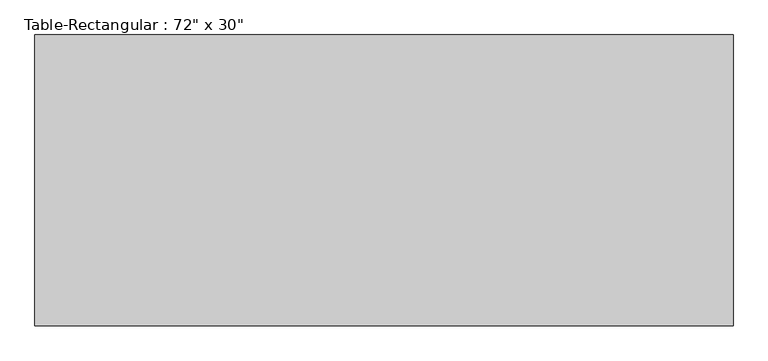
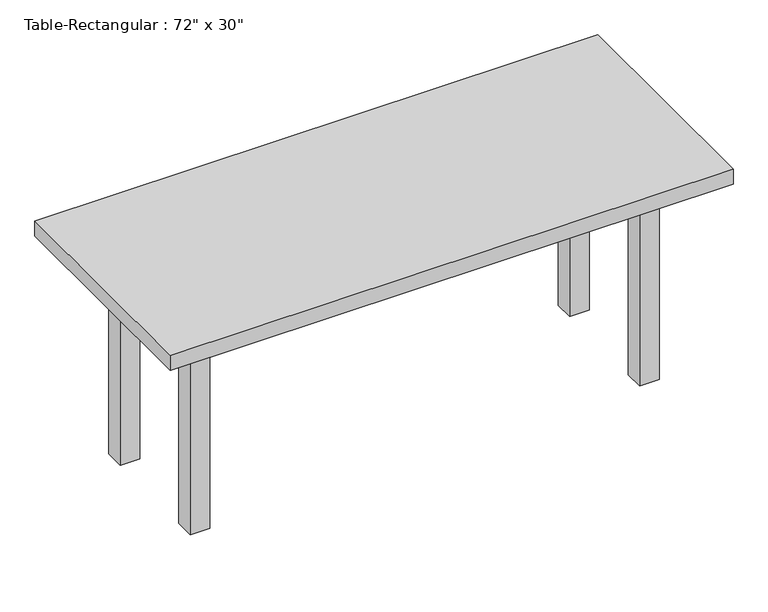
"""IFC4 building model written with IfcOpenShell, lengths in millimetres: furniture geometry."""

from ifc_helpers import new_model, si_unit, frame, origin, origin_with_axes, place, context, project, spatial, polyline, outline, extrude, source, transform, mapped, element, save


def furniture_a5b052b6(model_context):
    return source(origin(), model_context, "Body", "SweptSolid", [
        extrude(outline(polyline([(698.5, 190.5), (698.5, 165.1), (-698.5, 165.1), (-698.5, 190.5), (698.5, 190.5)])), frame((0.0, 0.0, 609.6), z_axis=(0.0, 0.0, 1.0), x_axis=(1.0, 0.0, 0.0)), (0.0, 0.0, 1.0), 101.6),
        extrude(outline(polyline([(698.5, -190.5), (-698.5, -190.5), (-698.5, -165.1), (698.5, -165.1), (698.5, -190.5)])), frame((0.0, 0.0, 609.6), z_axis=(0.0, 0.0, 1.0), x_axis=(1.0, 0.0, 0.0)), (0.0, 0.0, 1.0), 101.6),
        extrude(outline(polyline([(-711.2, -165.1), (-736.6, -165.1), (-736.6, 165.1), (-711.2, 165.1), (-711.2, -165.1)])), frame((0.0, 0.0, 609.6), z_axis=(0.0, 0.0, 1.0), x_axis=(1.0, 0.0, 0.0)), (0.0, 0.0, 1.0), 101.6),
        extrude(outline(polyline([(711.2, -165.1), (711.2, 165.1), (736.6, 165.1), (736.6, -165.1), (711.2, -165.1)])), frame((0.0, 0.0, 609.6), z_axis=(0.0, 0.0, 1.0), x_axis=(1.0, 0.0, 0.0)), (0.0, 0.0, 1.0), 101.6),
        extrude(outline(polyline([(914.4, 381.0), (914.4, -381.0), (-914.4, -381.0), (-914.4, 381.0), (914.4, 381.0)])), frame((0.0, 0.0, 711.2), z_axis=(0.0, 0.0, 1.0), x_axis=(1.0, 0.0, 0.0)), (0.0, 0.0, 1.0), 50.8),
        extrude(outline(polyline([(-698.5, 228.6), (-698.5, 165.1), (-762.0, 165.1), (-762.0, 228.6), (-698.5, 228.6)])), origin_with_axes(), (0.0, 0.0, 1.0), 711.2),
        extrude(outline(polyline([(698.5, 228.6), (762.0, 228.6), (762.0, 165.1), (698.5, 165.1), (698.5, 228.6)])), origin_with_axes(), (0.0, 0.0, 1.0), 711.2),
        extrude(outline(polyline([(-698.5, -228.6), (-762.0, -228.6), (-762.0, -165.1), (-698.5, -165.1), (-698.5, -228.6)])), origin_with_axes(), (0.0, 0.0, 1.0), 711.2),
        extrude(outline(polyline([(698.5, -228.6), (698.5, -165.1), (762.0, -165.1), (762.0, -228.6), (698.5, -228.6)])), origin_with_axes(), (0.0, 0.0, 1.0), 711.2),
    ])


if __name__ == "__main__":
    model = new_model("IFC4")
    model_context = context("Model", 3, world=origin())
    ifc_project = project(units=[si_unit("LENGTHUNIT", "METRE", prefix="MILLI")], contexts=[model_context])
    site = spatial("IfcSite", under=ifc_project)
    building = spatial("IfcBuilding", under=site)
    placement = place(None, origin())
    furniture_shape = furniture_a5b052b6(model_context)
    element("IfcFurniture", 1, ObjectType="Table-Rectangular : 72\" x 30\"", at=placement, inside=building, context=model_context, shape_type="MappedRepresentation", body=[
        mapped(furniture_shape, transform((0.0, 0.0, 0.0), x_axis=(1.0, 0.0, 0.0), y_axis=(0.0, 1.0, 0.0), z_axis=(0.0, 0.0, 1.0))),
    ])
    save(model, "model.ifc")

# Revit data of these elements
# Type "Table-Rectangular : 72\" x 30\""
#   Assembly Code = "E2020200"
#   Height = 2' - 6"
#   Length = 6' - 0"
#   Width = 2' - 6"
#   Base Material = Birch
#   Top Material = Birch
#   Default Elevation = 0
# Element 1 (IfcFurniture, "Table-Rectangular : 72\" x 30\"")
#   Materials on its faces: "Birch"
# Materials
#   "Birch": class "Wood", colour RGB 210 159 95, transparency 0, Description = "Betula Alleghaniensis", Cost = 0
